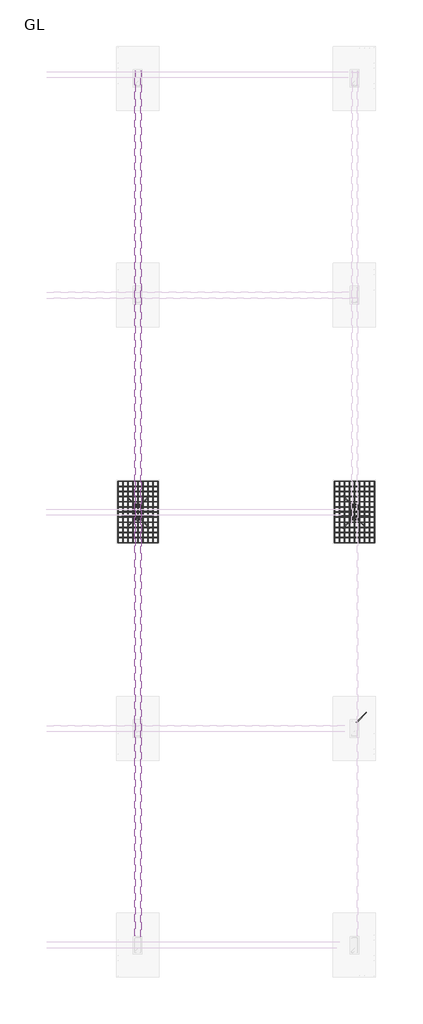
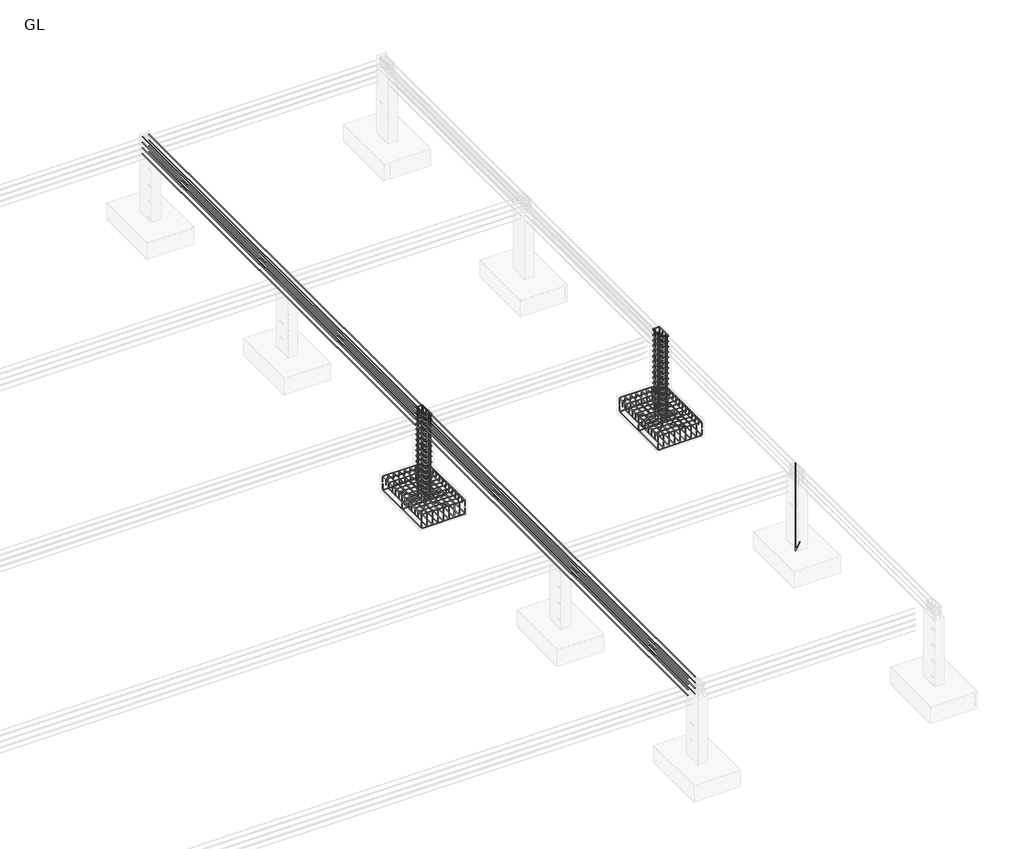
# One storey, part 12 of 16: 24 reinforcing bars.
"""IFC4 building model written with IfcOpenShell, lengths in millimetres."""

from ifc_helpers import new_model, si_unit, point, frame, origin, place, context, project, spatial, polyline, circle_curve, trimmed, segment, composite_curve, source, transform, mapped, element, save
from ifc_brep_helpers import swept_disk

model = new_model("IFC4")

# Units and contexts
model_context = context("Model", 3, world=origin())
ifc_project = project(units=[si_unit("LENGTHUNIT", "METRE", prefix="MILLI")], contexts=[model_context])

# Site, building, storey
site = spatial("IfcSite", under=ifc_project)
building = spatial("IfcBuilding", under=site)
storey = spatial("IfcBuildingStorey", under=building, Name="GL", Elevation=-1829.0)

# Reinforcing bars
placement = place(None, origin())
reinforcing_bar_shape = source(origin(), model_context, "Body", "SolidModel", [
    swept_disk(composite_curve([segment(polyline([(2141.0455621, -7223.1167521, -2089.0), (2141.0455621, -7223.1167521, -2213.0)]), True, "CONTINUOUS"), segment(trimmed(circle_curve(frame((2111.0455621, -7223.1167521, -2213.0), z_axis=(0.0, 1.0, 0.0), x_axis=(30.0, 0.0, 0.0)), 30.0), [point((2141.0455621, -7223.1167521, -2213.0))], [point((2111.0455621, -7223.1167521, -2243.0))], True, "CARTESIAN"), True, "CONTINUOUS"), segment(polyline([(2111.0455621, -7223.1167521, -2243.0), (1043.0455621, -7223.1167521, -2243.0)]), True, "CONTINUOUS"), segment(trimmed(circle_curve(frame((1043.0455621, -7223.1167521, -2213.0), z_axis=(0.0, 1.0, 0.0), x_axis=(0.0, 0.0, -30.0)), 30.0), [point((1043.0455621, -7223.1167521, -2243.0))], [point((1013.0455621, -7223.1167521, -2213.0))], True, "CARTESIAN"), True, "CONTINUOUS"), segment(polyline([(1013.0455621, -7223.1167521, -2213.0), (1013.0455621, -7223.1167521, -2089.0)]), True, "CONTINUOUS")], self_intersect=False), 6.0),
])
element("IfcReinforcingBar", 1, at=placement, inside=storey, context=model_context, shape_type="MappedRepresentation", body=[
    mapped(reinforcing_bar_shape, transform((0.0, 0.0, 0.0), x_axis=(1.0, 0.0, 0.0), y_axis=(0.0, 1.0, 0.0), z_axis=(0.0, 0.0, 1.0))),
    mapped(reinforcing_bar_shape, transform((0.0, -864.0, 0.0), x_axis=(1.0, 0.0, 0.0), y_axis=(0.0, 1.0, 0.0), z_axis=(0.0, 0.0, 1.0))),
    mapped(reinforcing_bar_shape, transform((0.0, -1728.0, 0.0), x_axis=(1.0, 0.0, 0.0), y_axis=(0.0, 1.0, 0.0), z_axis=(0.0, 0.0, 1.0))),
])
reinforcing_bar_2_shape = source(origin(), model_context, "Body", "SolidModel", [
    swept_disk(composite_curve([segment(polyline([(1013.0455621, -7223.1167521, -2022.436678), (1013.0455621, -7223.1167521, -1898.436678)]), True, "CONTINUOUS"), segment(trimmed(circle_curve(frame((1043.0455621, -7223.1167521, -1898.436678), z_axis=(0.0, 1.0, 0.0), x_axis=(-30.000000000000114, 0.0, 0.0)), 30.0), [point((1013.0455621, -7223.1167521, -1898.436678))], [point((1043.0455621, -7223.1167521, -1868.436678))], True, "CARTESIAN"), True, "CONTINUOUS"), segment(polyline([(1043.0455621, -7223.1167521, -1868.436678), (2111.0455621, -7223.1167521, -1868.436678)]), True, "CONTINUOUS"), segment(trimmed(circle_curve(frame((2111.0455621, -7223.1167521, -1898.436678), z_axis=(0.0, 1.0, 0.0), x_axis=(0.0, 0.0, 30.0)), 30.0), [point((2111.0455621, -7223.1167521, -1868.436678))], [point((2141.0455621, -7223.1167521, -1898.436678))], True, "CARTESIAN"), True, "CONTINUOUS"), segment(polyline([(2141.0455621, -7223.1167521, -1898.436678), (2141.0455621, -7223.1167521, -2022.436678)]), True, "CONTINUOUS")], self_intersect=False), 6.0),
])
element("IfcReinforcingBar", 2, at=placement, inside=storey, context=model_context, shape_type="MappedRepresentation", body=[
    mapped(reinforcing_bar_2_shape, transform((0.0, 0.0, 0.0), x_axis=(1.0, 0.0, 0.0), y_axis=(0.0, 1.0, 0.0), z_axis=(0.0, 0.0, 1.0))),
    mapped(reinforcing_bar_2_shape, transform((0.0, -144.0, 0.0), x_axis=(1.0, 0.0, 0.0), y_axis=(0.0, 1.0, 0.0), z_axis=(0.0, 0.0, 1.0))),
    mapped(reinforcing_bar_2_shape, transform((0.0, -288.0, 0.0), x_axis=(1.0, 0.0, 0.0), y_axis=(0.0, 1.0, 0.0), z_axis=(0.0, 0.0, 1.0))),
    mapped(reinforcing_bar_2_shape, transform((0.0, -432.0, 0.0), x_axis=(1.0, 0.0, 0.0), y_axis=(0.0, 1.0, 0.0), z_axis=(0.0, 0.0, 1.0))),
    mapped(reinforcing_bar_2_shape, transform((0.0, -576.0, 0.0), x_axis=(1.0, 0.0, 0.0), y_axis=(0.0, 1.0, 0.0), z_axis=(0.0, 0.0, 1.0))),
    mapped(reinforcing_bar_2_shape, transform((0.0, -720.0, 0.0), x_axis=(1.0, 0.0, 0.0), y_axis=(0.0, 1.0, 0.0), z_axis=(0.0, 0.0, 1.0))),
    mapped(reinforcing_bar_2_shape, transform((0.0, -864.0, 0.0), x_axis=(1.0, 0.0, 0.0), y_axis=(0.0, 1.0, 0.0), z_axis=(0.0, 0.0, 1.0))),
    mapped(reinforcing_bar_2_shape, transform((0.0, -1008.0, 0.0), x_axis=(1.0, 0.0, 0.0), y_axis=(0.0, 1.0, 0.0), z_axis=(0.0, 0.0, 1.0))),
    mapped(reinforcing_bar_2_shape, transform((0.0, -1152.0, 0.0), x_axis=(1.0, 0.0, 0.0), y_axis=(0.0, 1.0, 0.0), z_axis=(0.0, 0.0, 1.0))),
    mapped(reinforcing_bar_2_shape, transform((0.0, -1296.0, 0.0), x_axis=(1.0, 0.0, 0.0), y_axis=(0.0, 1.0, 0.0), z_axis=(0.0, 0.0, 1.0))),
    mapped(reinforcing_bar_2_shape, transform((0.0, -1440.0, 0.0), x_axis=(1.0, 0.0, 0.0), y_axis=(0.0, 1.0, 0.0), z_axis=(0.0, 0.0, 1.0))),
    mapped(reinforcing_bar_2_shape, transform((0.0, -1584.0, 0.0), x_axis=(1.0, 0.0, 0.0), y_axis=(0.0, 1.0, 0.0), z_axis=(0.0, 0.0, 1.0))),
    mapped(reinforcing_bar_2_shape, transform((0.0, -1728.0, 0.0), x_axis=(1.0, 0.0, 0.0), y_axis=(0.0, 1.0, 0.0), z_axis=(0.0, 0.0, 1.0))),
])
reinforcing_bar_3_shape = source(origin(), model_context, "Body", "SolidModel", [
    swept_disk(composite_curve([segment(polyline([(1013.0455621, -8951.1167521, -2027.5081232), (1013.0455621, -8951.1167521, -1903.5081232)]), True, "CONTINUOUS"), segment(trimmed(circle_curve(frame((1013.0455621, -8921.1167521, -1903.5081232), z_axis=(-1.0, 0.0, 0.0), x_axis=(0.0, -30.0, 0.0)), 30.0), [point((1013.0455621, -8951.1167521, -1903.5081232))], [point((1013.0455621, -8921.1167521, -1873.5081232))], True, "CARTESIAN"), True, "CONTINUOUS"), segment(polyline([(1013.0455621, -8921.1167521, -1873.5081232), (1013.0455621, -7253.1167521, -1873.5081232)]), True, "CONTINUOUS"), segment(trimmed(circle_curve(frame((1013.0455621, -7253.1167521, -1903.5081232), z_axis=(-1.0, 0.0, 0.0), x_axis=(0.0, 0.0, 30.0)), 30.0), [point((1013.0455621, -7253.1167521, -1873.5081232))], [point((1013.0455621, -7223.1167521, -1903.5081232))], True, "CARTESIAN"), True, "CONTINUOUS"), segment(polyline([(1013.0455621, -7223.1167521, -1903.5081232), (1013.0455621, -7223.1167521, -2027.5081232)]), True, "CONTINUOUS")], self_intersect=False), 6.0),
])
element("IfcReinforcingBar", 3, at=placement, inside=storey, context=model_context, shape_type="MappedRepresentation", body=[
    mapped(reinforcing_bar_3_shape, transform((0.0, 0.0, 0.0), x_axis=(1.0, 0.0, 0.0), y_axis=(0.0, 1.0, 0.0), z_axis=(0.0, 0.0, 1.0))),
    mapped(reinforcing_bar_3_shape, transform((141.0, 0.0, 0.0), x_axis=(1.0, 0.0, 0.0), y_axis=(0.0, 1.0, 0.0), z_axis=(0.0, 0.0, 1.0))),
    mapped(reinforcing_bar_3_shape, transform((282.0, 0.0, 0.0), x_axis=(1.0, 0.0, 0.0), y_axis=(0.0, 1.0, 0.0), z_axis=(0.0, 0.0, 1.0))),
    mapped(reinforcing_bar_3_shape, transform((423.0, 0.0, 0.0), x_axis=(1.0, 0.0, 0.0), y_axis=(0.0, 1.0, 0.0), z_axis=(0.0, 0.0, 1.0))),
    mapped(reinforcing_bar_3_shape, transform((564.0, 0.0, 0.0), x_axis=(1.0, 0.0, 0.0), y_axis=(0.0, 1.0, 0.0), z_axis=(0.0, 0.0, 1.0))),
    mapped(reinforcing_bar_3_shape, transform((705.0, 0.0, 0.0), x_axis=(1.0, 0.0, 0.0), y_axis=(0.0, 1.0, 0.0), z_axis=(0.0, 0.0, 1.0))),
    mapped(reinforcing_bar_3_shape, transform((846.0, 0.0, 0.0), x_axis=(1.0, 0.0, 0.0), y_axis=(0.0, 1.0, 0.0), z_axis=(0.0, 0.0, 1.0))),
    mapped(reinforcing_bar_3_shape, transform((987.0, 0.0, 0.0), x_axis=(1.0, 0.0, 0.0), y_axis=(0.0, 1.0, 0.0), z_axis=(0.0, 0.0, 1.0))),
    mapped(reinforcing_bar_3_shape, transform((1128.0, 0.0, 0.0), x_axis=(1.0, 0.0, 0.0), y_axis=(0.0, 1.0, 0.0), z_axis=(0.0, 0.0, 1.0))),
])
reinforcing_bar_4_shape = source(origin(), model_context, "Body", "SolidModel", [
    swept_disk(composite_curve([segment(polyline([(2141.0455621, -8951.1167521, -2080.6239909), (2141.0455621, -8951.1167521, -2204.6239909)]), True, "CONTINUOUS"), segment(trimmed(circle_curve(frame((2141.0455621, -8921.1167521, -2204.6239909), z_axis=(1.0, 0.0, 0.0), x_axis=(0.0, -30.0, 0.0)), 30.0), [point((2141.0455621, -8951.1167521, -2204.6239909))], [point((2141.0455621, -8921.1167521, -2234.6239909))], True, "CARTESIAN"), True, "CONTINUOUS"), segment(polyline([(2141.0455621, -8921.1167521, -2234.6239909), (2141.0455621, -7266.1421892, -2234.6239909)]), True, "CONTINUOUS"), segment(trimmed(circle_curve(frame((2141.0455621, -7266.1421892, -2204.6239909), z_axis=(1.0, 0.0, 0.0), x_axis=(0.0, 0.0, -30.0)), 30.0), [point((2141.0455621, -7266.1421892, -2234.6239909))], [point((2141.0455621, -7236.1421892, -2204.6239909))], True, "CARTESIAN"), True, "CONTINUOUS"), segment(polyline([(2141.0455621, -7236.1421892, -2204.6239909), (2141.0455621, -7236.1421892, -2080.6239909)]), True, "CONTINUOUS")], self_intersect=False), 6.0),
])
element("IfcReinforcingBar", 4, at=placement, inside=storey, context=model_context, shape_type="MappedRepresentation", body=[
    mapped(reinforcing_bar_4_shape, transform((0.0, 0.0, 0.0), x_axis=(1.0, 0.0, 0.0), y_axis=(0.0, 1.0, 0.0), z_axis=(0.0, 0.0, 1.0))),
    mapped(reinforcing_bar_4_shape, transform((-141.0, 0.0, 0.0), x_axis=(1.0, 0.0, 0.0), y_axis=(0.0, 1.0, 0.0), z_axis=(0.0, 0.0, 1.0))),
    mapped(reinforcing_bar_4_shape, transform((-282.0, 0.0, 0.0), x_axis=(1.0, 0.0, 0.0), y_axis=(0.0, 1.0, 0.0), z_axis=(0.0, 0.0, 1.0))),
    mapped(reinforcing_bar_4_shape, transform((-423.0, 0.0, 0.0), x_axis=(1.0, 0.0, 0.0), y_axis=(0.0, 1.0, 0.0), z_axis=(0.0, 0.0, 1.0))),
    mapped(reinforcing_bar_4_shape, transform((-564.0, 0.0, 0.0), x_axis=(1.0, 0.0, 0.0), y_axis=(0.0, 1.0, 0.0), z_axis=(0.0, 0.0, 1.0))),
    mapped(reinforcing_bar_4_shape, transform((-705.0, 0.0, 0.0), x_axis=(1.0, 0.0, 0.0), y_axis=(0.0, 1.0, 0.0), z_axis=(0.0, 0.0, 1.0))),
    mapped(reinforcing_bar_4_shape, transform((-846.0, 0.0, 0.0), x_axis=(1.0, 0.0, 0.0), y_axis=(0.0, 1.0, 0.0), z_axis=(0.0, 0.0, 1.0))),
    mapped(reinforcing_bar_4_shape, transform((-987.0, 0.0, 0.0), x_axis=(1.0, 0.0, 0.0), y_axis=(0.0, 1.0, 0.0), z_axis=(0.0, 0.0, 1.0))),
    mapped(reinforcing_bar_4_shape, transform((-1128.0, 0.0, 0.0), x_axis=(1.0, 0.0, 0.0), y_axis=(0.0, 1.0, 0.0), z_axis=(0.0, 0.0, 1.0))),
])
reinforcing_bar_5_shape = source(origin(), model_context, "Body", "SolidModel", [
    swept_disk(composite_curve([segment(polyline([(8237.0455621, -7223.1167521, -2089.0), (8237.0455621, -7223.1167521, -2213.0)]), True, "CONTINUOUS"), segment(trimmed(circle_curve(frame((8207.0455621, -7223.1167521, -2213.0), z_axis=(0.0, 1.0, 0.0), x_axis=(30.0, 0.0, 0.0)), 30.0), [point((8237.0455621, -7223.1167521, -2213.0))], [point((8207.0455621, -7223.1167521, -2243.0))], True, "CARTESIAN"), True, "CONTINUOUS"), segment(polyline([(8207.0455621, -7223.1167521, -2243.0), (7139.0455621, -7223.1167521, -2243.0)]), True, "CONTINUOUS"), segment(trimmed(circle_curve(frame((7139.0455621, -7223.1167521, -2213.0), z_axis=(0.0, 1.0, 0.0), x_axis=(0.0, 0.0, -30.0)), 30.0), [point((7139.0455621, -7223.1167521, -2243.0))], [point((7109.0455621, -7223.1167521, -2213.0))], True, "CARTESIAN"), True, "CONTINUOUS"), segment(polyline([(7109.0455621, -7223.1167521, -2213.0), (7109.0455621, -7223.1167521, -2089.0)]), True, "CONTINUOUS")], self_intersect=False), 6.0),
])
element("IfcReinforcingBar", 5, at=placement, inside=storey, context=model_context, shape_type="MappedRepresentation", body=[
    mapped(reinforcing_bar_5_shape, transform((0.0, 0.0, 0.0), x_axis=(1.0, 0.0, 0.0), y_axis=(0.0, 1.0, 0.0), z_axis=(0.0, 0.0, 1.0))),
    mapped(reinforcing_bar_5_shape, transform((0.0, -864.0, 0.0), x_axis=(1.0, 0.0, 0.0), y_axis=(0.0, 1.0, 0.0), z_axis=(0.0, 0.0, 1.0))),
    mapped(reinforcing_bar_5_shape, transform((0.0, -1728.0, 0.0), x_axis=(1.0, 0.0, 0.0), y_axis=(0.0, 1.0, 0.0), z_axis=(0.0, 0.0, 1.0))),
])
reinforcing_bar_6_shape = source(origin(), model_context, "Body", "SolidModel", [
    swept_disk(composite_curve([segment(polyline([(7109.0455621, -7223.1167521, -2022.436678), (7109.0455621, -7223.1167521, -1898.436678)]), True, "CONTINUOUS"), segment(trimmed(circle_curve(frame((7139.0455621, -7223.1167521, -1898.436678), z_axis=(0.0, 1.0, 0.0), x_axis=(-30.0, 0.0, 0.0)), 30.0), [point((7109.0455621, -7223.1167521, -1898.436678))], [point((7139.0455621, -7223.1167521, -1868.436678))], True, "CARTESIAN"), True, "CONTINUOUS"), segment(polyline([(7139.0455621, -7223.1167521, -1868.436678), (8207.0455621, -7223.1167521, -1868.436678)]), True, "CONTINUOUS"), segment(trimmed(circle_curve(frame((8207.0455621, -7223.1167521, -1898.436678), z_axis=(0.0, 1.0, 0.0), x_axis=(0.0, 0.0, 30.0)), 30.0), [point((8207.0455621, -7223.1167521, -1868.436678))], [point((8237.0455621, -7223.1167521, -1898.436678))], True, "CARTESIAN"), True, "CONTINUOUS"), segment(polyline([(8237.0455621, -7223.1167521, -1898.436678), (8237.0455621, -7223.1167521, -2022.436678)]), True, "CONTINUOUS")], self_intersect=False), 6.0),
])
element("IfcReinforcingBar", 6, at=placement, inside=storey, context=model_context, shape_type="MappedRepresentation", body=[
    mapped(reinforcing_bar_6_shape, transform((0.0, 0.0, 0.0), x_axis=(1.0, 0.0, 0.0), y_axis=(0.0, 1.0, 0.0), z_axis=(0.0, 0.0, 1.0))),
    mapped(reinforcing_bar_6_shape, transform((0.0, -144.0, 0.0), x_axis=(1.0, 0.0, 0.0), y_axis=(0.0, 1.0, 0.0), z_axis=(0.0, 0.0, 1.0))),
    mapped(reinforcing_bar_6_shape, transform((0.0, -288.0, 0.0), x_axis=(1.0, 0.0, 0.0), y_axis=(0.0, 1.0, 0.0), z_axis=(0.0, 0.0, 1.0))),
    mapped(reinforcing_bar_6_shape, transform((0.0, -432.0, 0.0), x_axis=(1.0, 0.0, 0.0), y_axis=(0.0, 1.0, 0.0), z_axis=(0.0, 0.0, 1.0))),
    mapped(reinforcing_bar_6_shape, transform((0.0, -576.0, 0.0), x_axis=(1.0, 0.0, 0.0), y_axis=(0.0, 1.0, 0.0), z_axis=(0.0, 0.0, 1.0))),
    mapped(reinforcing_bar_6_shape, transform((0.0, -720.0, 0.0), x_axis=(1.0, 0.0, 0.0), y_axis=(0.0, 1.0, 0.0), z_axis=(0.0, 0.0, 1.0))),
    mapped(reinforcing_bar_6_shape, transform((0.0, -864.0, 0.0), x_axis=(1.0, 0.0, 0.0), y_axis=(0.0, 1.0, 0.0), z_axis=(0.0, 0.0, 1.0))),
    mapped(reinforcing_bar_6_shape, transform((0.0, -1008.0, 0.0), x_axis=(1.0, 0.0, 0.0), y_axis=(0.0, 1.0, 0.0), z_axis=(0.0, 0.0, 1.0))),
    mapped(reinforcing_bar_6_shape, transform((0.0, -1152.0, 0.0), x_axis=(1.0, 0.0, 0.0), y_axis=(0.0, 1.0, 0.0), z_axis=(0.0, 0.0, 1.0))),
    mapped(reinforcing_bar_6_shape, transform((0.0, -1296.0, 0.0), x_axis=(1.0, 0.0, 0.0), y_axis=(0.0, 1.0, 0.0), z_axis=(0.0, 0.0, 1.0))),
    mapped(reinforcing_bar_6_shape, transform((0.0, -1440.0, 0.0), x_axis=(1.0, 0.0, 0.0), y_axis=(0.0, 1.0, 0.0), z_axis=(0.0, 0.0, 1.0))),
    mapped(reinforcing_bar_6_shape, transform((0.0, -1584.0, 0.0), x_axis=(1.0, 0.0, 0.0), y_axis=(0.0, 1.0, 0.0), z_axis=(0.0, 0.0, 1.0))),
    mapped(reinforcing_bar_6_shape, transform((0.0, -1728.0, 0.0), x_axis=(1.0, 0.0, 0.0), y_axis=(0.0, 1.0, 0.0), z_axis=(0.0, 0.0, 1.0))),
])
reinforcing_bar_7_shape = source(origin(), model_context, "Body", "SolidModel", [
    swept_disk(composite_curve([segment(polyline([(7109.0455621, -8951.1167521, -2027.5081232), (7109.0455621, -8951.1167521, -1903.5081232)]), True, "CONTINUOUS"), segment(trimmed(circle_curve(frame((7109.0455621, -8921.1167521, -1903.5081232), z_axis=(-1.0, 0.0, 0.0), x_axis=(0.0, -30.0, 0.0)), 30.0), [point((7109.0455621, -8951.1167521, -1903.5081232))], [point((7109.0455621, -8921.1167521, -1873.5081232))], True, "CARTESIAN"), True, "CONTINUOUS"), segment(polyline([(7109.0455621, -8921.1167521, -1873.5081232), (7109.0455621, -7253.1167521, -1873.5081232)]), True, "CONTINUOUS"), segment(trimmed(circle_curve(frame((7109.0455621, -7253.1167521, -1903.5081232), z_axis=(-1.0, 0.0, 0.0), x_axis=(0.0, 0.0, 30.0)), 30.0), [point((7109.0455621, -7253.1167521, -1873.5081232))], [point((7109.0455621, -7223.1167521, -1903.5081232))], True, "CARTESIAN"), True, "CONTINUOUS"), segment(polyline([(7109.0455621, -7223.1167521, -1903.5081232), (7109.0455621, -7223.1167521, -2027.5081232)]), True, "CONTINUOUS")], self_intersect=False), 6.0),
])
element("IfcReinforcingBar", 7, at=placement, inside=storey, context=model_context, shape_type="MappedRepresentation", body=[
    mapped(reinforcing_bar_7_shape, transform((0.0, 0.0, 0.0), x_axis=(1.0, 0.0, 0.0), y_axis=(0.0, 1.0, 0.0), z_axis=(0.0, 0.0, 1.0))),
    mapped(reinforcing_bar_7_shape, transform((141.0, 0.0, 0.0), x_axis=(1.0, 0.0, 0.0), y_axis=(0.0, 1.0, 0.0), z_axis=(0.0, 0.0, 1.0))),
    mapped(reinforcing_bar_7_shape, transform((282.0, 0.0, 0.0), x_axis=(1.0, 0.0, 0.0), y_axis=(0.0, 1.0, 0.0), z_axis=(0.0, 0.0, 1.0))),
    mapped(reinforcing_bar_7_shape, transform((423.0, 0.0, 0.0), x_axis=(1.0, 0.0, 0.0), y_axis=(0.0, 1.0, 0.0), z_axis=(0.0, 0.0, 1.0))),
    mapped(reinforcing_bar_7_shape, transform((564.0, 0.0, 0.0), x_axis=(1.0, 0.0, 0.0), y_axis=(0.0, 1.0, 0.0), z_axis=(0.0, 0.0, 1.0))),
    mapped(reinforcing_bar_7_shape, transform((705.0, 0.0, 0.0), x_axis=(1.0, 0.0, 0.0), y_axis=(0.0, 1.0, 0.0), z_axis=(0.0, 0.0, 1.0))),
    mapped(reinforcing_bar_7_shape, transform((846.0, 0.0, 0.0), x_axis=(1.0, 0.0, 0.0), y_axis=(0.0, 1.0, 0.0), z_axis=(0.0, 0.0, 1.0))),
    mapped(reinforcing_bar_7_shape, transform((987.0, 0.0, 0.0), x_axis=(1.0, 0.0, 0.0), y_axis=(0.0, 1.0, 0.0), z_axis=(0.0, 0.0, 1.0))),
    mapped(reinforcing_bar_7_shape, transform((1128.0, 0.0, 0.0), x_axis=(1.0, 0.0, 0.0), y_axis=(0.0, 1.0, 0.0), z_axis=(0.0, 0.0, 1.0))),
])
reinforcing_bar_8_shape = source(origin(), model_context, "Body", "SolidModel", [
    swept_disk(composite_curve([segment(polyline([(8237.0455621, -8951.1167521, -2080.6239909), (8237.0455621, -8951.1167521, -2204.6239909)]), True, "CONTINUOUS"), segment(trimmed(circle_curve(frame((8237.0455621, -8921.1167521, -2204.6239909), z_axis=(1.0, 0.0, 0.0), x_axis=(0.0, -30.0, 0.0)), 30.0), [point((8237.0455621, -8951.1167521, -2204.6239909))], [point((8237.0455621, -8921.1167521, -2234.6239909))], True, "CARTESIAN"), True, "CONTINUOUS"), segment(polyline([(8237.0455621, -8921.1167521, -2234.6239909), (8237.0455621, -7266.1421892, -2234.6239909)]), True, "CONTINUOUS"), segment(trimmed(circle_curve(frame((8237.0455621, -7266.1421892, -2204.6239909), z_axis=(1.0, 0.0, 0.0), x_axis=(0.0, 0.0, -30.0)), 30.0), [point((8237.0455621, -7266.1421892, -2234.6239909))], [point((8237.0455621, -7236.1421892, -2204.6239909))], True, "CARTESIAN"), True, "CONTINUOUS"), segment(polyline([(8237.0455621, -7236.1421892, -2204.6239909), (8237.0455621, -7236.1421892, -2080.6239909)]), True, "CONTINUOUS")], self_intersect=False), 6.0),
])
element("IfcReinforcingBar", 8, at=placement, inside=storey, context=model_context, shape_type="MappedRepresentation", body=[
    mapped(reinforcing_bar_8_shape, transform((0.0, 0.0, 0.0), x_axis=(1.0, 0.0, 0.0), y_axis=(0.0, 1.0, 0.0), z_axis=(0.0, 0.0, 1.0))),
    mapped(reinforcing_bar_8_shape, transform((-141.0, 0.0, 0.0), x_axis=(1.0, 0.0, 0.0), y_axis=(0.0, 1.0, 0.0), z_axis=(0.0, 0.0, 1.0))),
    mapped(reinforcing_bar_8_shape, transform((-282.0, 0.0, 0.0), x_axis=(1.0, 0.0, 0.0), y_axis=(0.0, 1.0, 0.0), z_axis=(0.0, 0.0, 1.0))),
    mapped(reinforcing_bar_8_shape, transform((-423.0, 0.0, 0.0), x_axis=(1.0, 0.0, 0.0), y_axis=(0.0, 1.0, 0.0), z_axis=(0.0, 0.0, 1.0))),
    mapped(reinforcing_bar_8_shape, transform((-564.0, 0.0, 0.0), x_axis=(1.0, 0.0, 0.0), y_axis=(0.0, 1.0, 0.0), z_axis=(0.0, 0.0, 1.0))),
    mapped(reinforcing_bar_8_shape, transform((-705.0, 0.0, 0.0), x_axis=(1.0, 0.0, 0.0), y_axis=(0.0, 1.0, 0.0), z_axis=(0.0, 0.0, 1.0))),
    mapped(reinforcing_bar_8_shape, transform((-846.0, 0.0, 0.0), x_axis=(1.0, 0.0, 0.0), y_axis=(0.0, 1.0, 0.0), z_axis=(0.0, 0.0, 1.0))),
    mapped(reinforcing_bar_8_shape, transform((-987.0, 0.0, 0.0), x_axis=(1.0, 0.0, 0.0), y_axis=(0.0, 1.0, 0.0), z_axis=(0.0, 0.0, 1.0))),
    mapped(reinforcing_bar_8_shape, transform((-1128.0, 0.0, 0.0), x_axis=(1.0, 0.0, 0.0), y_axis=(0.0, 1.0, 0.0), z_axis=(0.0, 0.0, 1.0))),
])
reinforcing_bar_9_shape = source(origin(), model_context, "Body", "SolidModel", [
    swept_disk(composite_curve([segment(polyline([(7680.5135995, -8162.2223078, -1793.0), (7592.8323586, -8249.9035486, -1793.0)]), True, "CONTINUOUS"), segment(trimmed(circle_curve(frame((7614.0455621, -8271.1167521, -1793.0), z_axis=(0.0, 0.0, 1.0), x_axis=(-21.213203500000418, 21.213203500001327, 0.0)), 30.0), [point((7592.8323586, -8249.9035486, -1793.0))], [point((7614.0455621, -8301.1167521, -1793.0))], True, "CARTESIAN"), True, "CONTINUOUS"), segment(polyline([(7614.0455621, -8301.1167521, -1793.0), (7732.0455621, -8301.1167521, -1793.0)]), True, "CONTINUOUS"), segment(trimmed(circle_curve(frame((7732.0455621, -8271.1167521, -1793.0), z_axis=(0.0, 0.0, 1.0), x_axis=(0.0, -30.0, 0.0)), 30.0), [point((7732.0455621, -8301.1167521, -1793.0))], [point((7762.0455621, -8271.1167521, -1793.0))], True, "CARTESIAN"), True, "CONTINUOUS"), segment(polyline([(7762.0455621, -8271.1167521, -1793.0), (7762.0455621, -7903.1167521, -1793.0)]), True, "CONTINUOUS"), segment(trimmed(circle_curve(frame((7732.1135038, -7903.1167521, -1795.0178916), z_axis=(-0.06726305234213417, 0.0, 0.9977352764083365), x_axis=(29.93205829999988, 0.0, 2.0178915999999845)), 30.0), [point((7762.0455621, -7903.1167521, -1793.0))], [point((7732.1135038, -7873.1167521, -1795.0178916))], True, "CARTESIAN"), True, "CONTINUOUS"), segment(polyline([(7732.1135038, -7873.1167521, -1795.0178916), (7613.9776204, -7873.1167521, -1802.9821084)]), True, "CONTINUOUS"), segment(trimmed(circle_curve(frame((7613.9776204, -7903.1167521, -1802.9821084), z_axis=(-0.06726305234213417, 0.0, 0.9977352764083365), x_axis=(0.0, 30.0, 0.0)), 30.0), [point((7613.9776204, -7873.1167521, -1802.9821084))], [point((7584.0455621, -7903.1167521, -1805.0))], True, "CARTESIAN"), True, "CONTINUOUS"), segment(polyline([(7584.0455621, -7903.1167521, -1805.0), (7584.0455621, -8271.1167521, -1805.0)]), True, "CONTINUOUS"), segment(trimmed(circle_curve(frame((7614.0455621, -8271.1167521, -1805.0), z_axis=(0.0, 0.0, 1.0), x_axis=(-30.0, 0.0, 0.0)), 30.0), [point((7584.0455621, -8271.1167521, -1805.0))], [point((7635.2587655, -8292.3299555, -1805.0))], True, "CARTESIAN"), True, "CONTINUOUS"), segment(polyline([(7635.2587655, -8292.3299555, -1805.0), (7722.9400064, -8204.6487146, -1805.0)]), True, "CONTINUOUS")], self_intersect=False), 6.0),
])
element("IfcReinforcingBar", 9, at=placement, inside=storey, context=model_context, shape_type="MappedRepresentation", body=[
    mapped(reinforcing_bar_9_shape, transform((0.0, 0.0, 0.0), x_axis=(1.0, 0.0, 0.0), y_axis=(0.0, 1.0, 0.0), z_axis=(0.0, 0.0, 1.0))),
    mapped(reinforcing_bar_9_shape, transform((0.0, 0.0, 144.8571429), x_axis=(1.0, 0.0, 0.0), y_axis=(0.0, 1.0, 0.0), z_axis=(0.0, 0.0, 1.0))),
    mapped(reinforcing_bar_9_shape, transform((0.0, 0.0, 289.7142857), x_axis=(1.0, 0.0, 0.0), y_axis=(0.0, 1.0, 0.0), z_axis=(0.0, 0.0, 1.0))),
    mapped(reinforcing_bar_9_shape, transform((0.0, 0.0, 434.5714286), x_axis=(1.0, 0.0, 0.0), y_axis=(0.0, 1.0, 0.0), z_axis=(0.0, 0.0, 1.0))),
    mapped(reinforcing_bar_9_shape, transform((0.0, 0.0, 579.4285714), x_axis=(1.0, 0.0, 0.0), y_axis=(0.0, 1.0, 0.0), z_axis=(0.0, 0.0, 1.0))),
    mapped(reinforcing_bar_9_shape, transform((0.0, 0.0, 724.2857143), x_axis=(1.0, 0.0, 0.0), y_axis=(0.0, 1.0, 0.0), z_axis=(0.0, 0.0, 1.0))),
    mapped(reinforcing_bar_9_shape, transform((0.0, 0.0, 869.1428571), x_axis=(1.0, 0.0, 0.0), y_axis=(0.0, 1.0, 0.0), z_axis=(0.0, 0.0, 1.0))),
    mapped(reinforcing_bar_9_shape, transform((0.0, 0.0, 1014.0), x_axis=(1.0, 0.0, 0.0), y_axis=(0.0, 1.0, 0.0), z_axis=(0.0, 0.0, 1.0))),
    mapped(reinforcing_bar_9_shape, transform((0.0, 0.0, 1158.8571429), x_axis=(1.0, 0.0, 0.0), y_axis=(0.0, 1.0, 0.0), z_axis=(0.0, 0.0, 1.0))),
    mapped(reinforcing_bar_9_shape, transform((0.0, 0.0, 1303.7142857), x_axis=(1.0, 0.0, 0.0), y_axis=(0.0, 1.0, 0.0), z_axis=(0.0, 0.0, 1.0))),
    mapped(reinforcing_bar_9_shape, transform((0.0, 0.0, 1448.5714286), x_axis=(1.0, 0.0, 0.0), y_axis=(0.0, 1.0, 0.0), z_axis=(0.0, 0.0, 1.0))),
    mapped(reinforcing_bar_9_shape, transform((0.0, 0.0, 1593.4285714), x_axis=(1.0, 0.0, 0.0), y_axis=(0.0, 1.0, 0.0), z_axis=(0.0, 0.0, 1.0))),
    mapped(reinforcing_bar_9_shape, transform((0.0, 0.0, 1738.2857143), x_axis=(1.0, 0.0, 0.0), y_axis=(0.0, 1.0, 0.0), z_axis=(0.0, 0.0, 1.0))),
    mapped(reinforcing_bar_9_shape, transform((0.0, 0.0, 1883.1428571), x_axis=(1.0, 0.0, 0.0), y_axis=(0.0, 1.0, 0.0), z_axis=(0.0, 0.0, 1.0))),
    mapped(reinforcing_bar_9_shape, transform((0.0, 0.0, 2028.0), x_axis=(1.0, 0.0, 0.0), y_axis=(0.0, 1.0, 0.0), z_axis=(0.0, 0.0, 1.0))),
])
element("IfcReinforcingBar", 10, at=placement, inside=storey, context=model_context, shape_type="SolidModel", body=[
    swept_disk(composite_curve([segment(polyline([(7615.9357768, -8272.0642439, 241.0), (7615.9357768, -8272.0642439, -2129.0)]), True, "CONTINUOUS"), segment(trimmed(circle_curve(frame((7594.7225734, -8293.2774473, -2129.0), z_axis=(-0.7071067811865187, 0.7071067811865764, 0.0), x_axis=(21.213203399999657, 21.213203400000566, 0.0)), 30.0), [point((7615.9357768, -8272.0642439, -2129.0))], [point((7594.7225734, -8293.2774473, -2159.0))], True, "CARTESIAN"), True, "CONTINUOUS"), segment(polyline([(7594.7225734, -8293.2774473, -2159.0), (7347.2352, -8540.7648207, -2159.0)]), True, "CONTINUOUS")], self_intersect=False), 6.0),
])
element("IfcReinforcingBar", 11, at=placement, inside=storey, context=model_context, shape_type="SolidModel", body=[
    swept_disk(composite_curve([segment(polyline([(7615.9357768, -7902.1692603, 241.0), (7615.9357768, -7902.1692603, -2129.0)]), True, "CONTINUOUS"), segment(trimmed(circle_curve(frame((7594.7225734, -7880.9560568, -2129.0), z_axis=(0.7071067811865218, 0.7071067811865733, 0.0), x_axis=(21.213203399999657, -21.213203500000418, 0.0)), 30.0), [point((7615.9357768, -7902.1692603, -2129.0))], [point((7594.7225734, -7880.9560568, -2159.0))], True, "CARTESIAN"), True, "CONTINUOUS"), segment(polyline([(7594.7225734, -7880.9560568, -2159.0), (7347.2352, -7633.4686834, -2159.0)]), True, "CONTINUOUS")], self_intersect=False), 6.0),
])
element("IfcReinforcingBar", 12, at=placement, inside=storey, context=model_context, shape_type="SolidModel", body=[
    swept_disk(composite_curve([segment(polyline([(7730.1553473, -8272.0642439, 241.0), (7730.1553473, -8272.0642439, -2129.0)]), True, "CONTINUOUS"), segment(trimmed(circle_curve(frame((7751.3685508, -8293.2774473, -2129.0), z_axis=(-0.7071067811865248, -0.7071067811865703, 0.0), x_axis=(-21.21320349999951, 21.213203400000566, 0.0)), 30.0), [point((7730.1553473, -8272.0642439, -2129.0))], [point((7751.3685508, -8293.2774473, -2159.0))], True, "CARTESIAN"), True, "CONTINUOUS"), segment(polyline([(7751.3685508, -8293.2774473, -2159.0), (7998.8559242, -8540.7648207, -2159.0)]), True, "CONTINUOUS")], self_intersect=False), 6.0),
])
reinforcing_bar_10_shape = source(origin(), model_context, "Body", "SolidModel", [
    swept_disk(composite_curve([segment(polyline([(7615.9357768, -8194.9117405, 241.0), (7615.9357768, -8194.9117405, -2129.0)]), True, "CONTINUOUS"), segment(trimmed(circle_curve(frame((7585.9357768, -8194.9117405, -2129.0), z_axis=(0.0, 1.0, 0.0), x_axis=(30.0, 0.0, 0.0)), 30.0), [point((7615.9357768, -8194.9117405, -2129.0))], [point((7585.9357768, -8194.9117405, -2159.0))], True, "CARTESIAN"), True, "CONTINUOUS"), segment(polyline([(7585.9357768, -8194.9117405, -2159.0), (7235.9357768, -8194.9117405, -2159.0)]), True, "CONTINUOUS")], self_intersect=False), 6.0),
])
element("IfcReinforcingBar", 13, at=placement, inside=storey, context=model_context, shape_type="MappedRepresentation", body=[
    mapped(reinforcing_bar_10_shape, transform((0.0, 0.0, 0.0), x_axis=(1.0, 0.0, 0.0), y_axis=(0.0, 1.0, 0.0), z_axis=(0.0, 0.0, 1.0))),
    mapped(reinforcing_bar_10_shape, transform((0.0, 123.5823926, 0.0), x_axis=(1.0, 0.0, 0.0), y_axis=(0.0, 1.0, 0.0), z_axis=(0.0, 0.0, 1.0))),
    mapped(reinforcing_bar_10_shape, transform((0.0, 247.1647853, 0.0), x_axis=(1.0, 0.0, 0.0), y_axis=(0.0, 1.0, 0.0), z_axis=(0.0, 0.0, 1.0))),
])
reinforcing_bar_11_shape = source(origin(), model_context, "Body", "SolidModel", [
    swept_disk(composite_curve([segment(polyline([(7730.1553473, -8194.9117405, 241.0), (7730.1553473, -8194.9117405, -2129.0)]), True, "CONTINUOUS"), segment(trimmed(circle_curve(frame((7760.1553473, -8194.9117405, -2129.0), z_axis=(0.0, -1.0, 0.0), x_axis=(-30.0, 0.0, 0.0)), 30.0), [point((7730.1553473, -8194.9117405, -2129.0))], [point((7760.1553473, -8194.9117405, -2159.0))], True, "CARTESIAN"), True, "CONTINUOUS"), segment(polyline([(7760.1553473, -8194.9117405, -2159.0), (8110.1553473, -8194.9117405, -2159.0)]), True, "CONTINUOUS")], self_intersect=False), 6.0),
])
element("IfcReinforcingBar", 14, at=placement, inside=storey, context=model_context, shape_type="MappedRepresentation", body=[
    mapped(reinforcing_bar_11_shape, transform((0.0, 0.0, 0.0), x_axis=(1.0, 0.0, 0.0), y_axis=(0.0, 1.0, 0.0), z_axis=(0.0, 0.0, 1.0))),
    mapped(reinforcing_bar_11_shape, transform((0.0, 123.5823926, 0.0), x_axis=(1.0, 0.0, 0.0), y_axis=(0.0, 1.0, 0.0), z_axis=(0.0, 0.0, 1.0))),
    mapped(reinforcing_bar_11_shape, transform((0.0, 247.1647853, 0.0), x_axis=(1.0, 0.0, 0.0), y_axis=(0.0, 1.0, 0.0), z_axis=(0.0, 0.0, 1.0))),
])
element("IfcReinforcingBar", 15, at=placement, inside=storey, context=model_context, shape_type="SolidModel", body=[
    swept_disk(composite_curve([segment(polyline([(7730.1553473, -13998.1692603, 241.0), (7730.1553473, -13998.1692603, -2129.0)]), True, "CONTINUOUS"), segment(trimmed(circle_curve(frame((7751.3685508, -13976.9560568, -2129.0), z_axis=(0.7071067811865157, -0.7071067811865794, 0.0), x_axis=(-21.21320349999951, -21.21320349999951, 0.0)), 30.0), [point((7730.1553473, -13998.1692603, -2129.0))], [point((7751.3685508, -13976.9560568, -2159.0))], True, "CARTESIAN"), True, "CONTINUOUS"), segment(polyline([(7751.3685508, -13976.9560568, -2159.0), (7998.8559242, -13729.4686834, -2159.0)]), True, "CONTINUOUS")], self_intersect=False), 6.0),
])
reinforcing_bar_12_shape = source(origin(), model_context, "Body", "SolidModel", [
    swept_disk(composite_curve([segment(polyline([(1584.5135995, -8162.2223078, -1793.0), (1496.8323586, -8249.9035486, -1793.0)]), True, "CONTINUOUS"), segment(trimmed(circle_curve(frame((1518.0455621, -8271.1167521, -1793.0), z_axis=(0.0, 0.0, 1.0), x_axis=(-21.21320350000019, 21.213203500001327, 0.0)), 30.0), [point((1496.8323586, -8249.9035486, -1793.0))], [point((1518.0455621, -8301.1167521, -1793.0))], True, "CARTESIAN"), True, "CONTINUOUS"), segment(polyline([(1518.0455621, -8301.1167521, -1793.0), (1636.0455621, -8301.1167521, -1793.0)]), True, "CONTINUOUS"), segment(trimmed(circle_curve(frame((1636.0455621, -8271.1167521, -1793.0), z_axis=(0.0, 0.0, 1.0), x_axis=(0.0, -30.0, 0.0)), 30.0), [point((1636.0455621, -8301.1167521, -1793.0))], [point((1666.0455621, -8271.1167521, -1793.0))], True, "CARTESIAN"), True, "CONTINUOUS"), segment(polyline([(1666.0455621, -8271.1167521, -1793.0), (1666.0455621, -7903.1167521, -1793.0)]), True, "CONTINUOUS"), segment(trimmed(circle_curve(frame((1636.1135038, -7903.1167521, -1795.0178916), z_axis=(-0.06726305234213417, 0.0, 0.9977352764083365), x_axis=(29.932058300000108, 0.0, 2.0178915999999845)), 30.0), [point((1666.0455621, -7903.1167521, -1793.0))], [point((1636.1135038, -7873.1167521, -1795.0178916))], True, "CARTESIAN"), True, "CONTINUOUS"), segment(polyline([(1636.1135038, -7873.1167521, -1795.0178916), (1517.9776204, -7873.1167521, -1802.9821084)]), True, "CONTINUOUS"), segment(trimmed(circle_curve(frame((1517.9776204, -7903.1167521, -1802.9821084), z_axis=(-0.06726305234213417, 0.0, 0.9977352764083365), x_axis=(0.0, 30.0, 0.0)), 30.0), [point((1517.9776204, -7873.1167521, -1802.9821084))], [point((1488.0455621, -7903.1167521, -1805.0))], True, "CARTESIAN"), True, "CONTINUOUS"), segment(polyline([(1488.0455621, -7903.1167521, -1805.0), (1488.0455621, -8271.1167521, -1805.0)]), True, "CONTINUOUS"), segment(trimmed(circle_curve(frame((1518.0455621, -8271.1167521, -1805.0), z_axis=(0.0, 0.0, 1.0), x_axis=(-30.0, 0.0, 0.0)), 30.0), [point((1488.0455621, -8271.1167521, -1805.0))], [point((1539.2587655, -8292.3299555, -1805.0))], True, "CARTESIAN"), True, "CONTINUOUS"), segment(polyline([(1539.2587655, -8292.3299555, -1805.0), (1626.9400064, -8204.6487146, -1805.0)]), True, "CONTINUOUS")], self_intersect=False), 6.0),
])
element("IfcReinforcingBar", 16, at=placement, inside=storey, context=model_context, shape_type="MappedRepresentation", body=[
    mapped(reinforcing_bar_12_shape, transform((0.0, 0.0, 0.0), x_axis=(1.0, 0.0, 0.0), y_axis=(0.0, 1.0, 0.0), z_axis=(0.0, 0.0, 1.0))),
    mapped(reinforcing_bar_12_shape, transform((0.0, 0.0, 144.8571429), x_axis=(1.0, 0.0, 0.0), y_axis=(0.0, 1.0, 0.0), z_axis=(0.0, 0.0, 1.0))),
    mapped(reinforcing_bar_12_shape, transform((0.0, 0.0, 289.7142857), x_axis=(1.0, 0.0, 0.0), y_axis=(0.0, 1.0, 0.0), z_axis=(0.0, 0.0, 1.0))),
    mapped(reinforcing_bar_12_shape, transform((0.0, 0.0, 434.5714286), x_axis=(1.0, 0.0, 0.0), y_axis=(0.0, 1.0, 0.0), z_axis=(0.0, 0.0, 1.0))),
    mapped(reinforcing_bar_12_shape, transform((0.0, 0.0, 579.4285714), x_axis=(1.0, 0.0, 0.0), y_axis=(0.0, 1.0, 0.0), z_axis=(0.0, 0.0, 1.0))),
    mapped(reinforcing_bar_12_shape, transform((0.0, 0.0, 724.2857143), x_axis=(1.0, 0.0, 0.0), y_axis=(0.0, 1.0, 0.0), z_axis=(0.0, 0.0, 1.0))),
    mapped(reinforcing_bar_12_shape, transform((0.0, 0.0, 869.1428571), x_axis=(1.0, 0.0, 0.0), y_axis=(0.0, 1.0, 0.0), z_axis=(0.0, 0.0, 1.0))),
    mapped(reinforcing_bar_12_shape, transform((0.0, 0.0, 1014.0), x_axis=(1.0, 0.0, 0.0), y_axis=(0.0, 1.0, 0.0), z_axis=(0.0, 0.0, 1.0))),
    mapped(reinforcing_bar_12_shape, transform((0.0, 0.0, 1158.8571429), x_axis=(1.0, 0.0, 0.0), y_axis=(0.0, 1.0, 0.0), z_axis=(0.0, 0.0, 1.0))),
    mapped(reinforcing_bar_12_shape, transform((0.0, 0.0, 1303.7142857), x_axis=(1.0, 0.0, 0.0), y_axis=(0.0, 1.0, 0.0), z_axis=(0.0, 0.0, 1.0))),
    mapped(reinforcing_bar_12_shape, transform((0.0, 0.0, 1448.5714286), x_axis=(1.0, 0.0, 0.0), y_axis=(0.0, 1.0, 0.0), z_axis=(0.0, 0.0, 1.0))),
    mapped(reinforcing_bar_12_shape, transform((0.0, 0.0, 1593.4285714), x_axis=(1.0, 0.0, 0.0), y_axis=(0.0, 1.0, 0.0), z_axis=(0.0, 0.0, 1.0))),
    mapped(reinforcing_bar_12_shape, transform((0.0, 0.0, 1738.2857143), x_axis=(1.0, 0.0, 0.0), y_axis=(0.0, 1.0, 0.0), z_axis=(0.0, 0.0, 1.0))),
    mapped(reinforcing_bar_12_shape, transform((0.0, 0.0, 1883.1428571), x_axis=(1.0, 0.0, 0.0), y_axis=(0.0, 1.0, 0.0), z_axis=(0.0, 0.0, 1.0))),
    mapped(reinforcing_bar_12_shape, transform((0.0, 0.0, 2028.0), x_axis=(1.0, 0.0, 0.0), y_axis=(0.0, 1.0, 0.0), z_axis=(0.0, 0.0, 1.0))),
])
element("IfcReinforcingBar", 17, at=placement, inside=storey, context=model_context, shape_type="SolidModel", body=[
    swept_disk(composite_curve([segment(polyline([(1519.9357768, -8272.0642439, 241.0), (1519.9357768, -8272.0642439, -2129.0)]), True, "CONTINUOUS"), segment(trimmed(circle_curve(frame((1498.7225734, -8293.2774473, -2129.0), z_axis=(-0.7071067811865187, 0.7071067811865764, 0.0), x_axis=(21.213203399999884, 21.213203400000566, 0.0)), 30.0), [point((1519.9357768, -8272.0642439, -2129.0))], [point((1498.7225734, -8293.2774473, -2159.0))], True, "CARTESIAN"), True, "CONTINUOUS"), segment(polyline([(1498.7225734, -8293.2774473, -2159.0), (1251.2352, -8540.7648207, -2159.0)]), True, "CONTINUOUS")], self_intersect=False), 6.0),
])
element("IfcReinforcingBar", 18, at=placement, inside=storey, context=model_context, shape_type="SolidModel", body=[
    swept_disk(composite_curve([segment(polyline([(1519.9357768, -7902.1692603, 241.0), (1519.9357768, -7902.1692603, -2129.0)]), True, "CONTINUOUS"), segment(trimmed(circle_curve(frame((1498.7225734, -7880.9560568, -2129.0), z_axis=(0.7071067811865218, 0.7071067811865733, 0.0), x_axis=(21.213203399999884, -21.213203500000418, 0.0)), 30.0), [point((1519.9357768, -7902.1692603, -2129.0))], [point((1498.7225734, -7880.9560568, -2159.0))], True, "CARTESIAN"), True, "CONTINUOUS"), segment(polyline([(1498.7225734, -7880.9560568, -2159.0), (1251.2352, -7633.4686834, -2159.0)]), True, "CONTINUOUS")], self_intersect=False), 6.0),
])
element("IfcReinforcingBar", 19, at=placement, inside=storey, context=model_context, shape_type="SolidModel", body=[
    swept_disk(composite_curve([segment(polyline([(1634.1553473, -8272.0642439, 241.0), (1634.1553473, -8272.0642439, -2129.0)]), True, "CONTINUOUS"), segment(trimmed(circle_curve(frame((1655.3685508, -8293.2774473, -2129.0), z_axis=(-0.7071067811865248, -0.7071067811865703, 0.0), x_axis=(-21.21320350000019, 21.213203400000566, 0.0)), 30.0), [point((1634.1553473, -8272.0642439, -2129.0))], [point((1655.3685508, -8293.2774473, -2159.0))], True, "CARTESIAN"), True, "CONTINUOUS"), segment(polyline([(1655.3685508, -8293.2774473, -2159.0), (1902.8559242, -8540.7648207, -2159.0)]), True, "CONTINUOUS")], self_intersect=False), 6.0),
])
element("IfcReinforcingBar", 20, at=placement, inside=storey, context=model_context, shape_type="SolidModel", body=[
    swept_disk(composite_curve([segment(polyline([(1634.1553473, -7902.1692603, 241.0), (1634.1553473, -7902.1692603, -2129.0)]), True, "CONTINUOUS"), segment(trimmed(circle_curve(frame((1655.3685508, -7880.9560568, -2129.0), z_axis=(0.7071067811865157, -0.7071067811865794, 0.0), x_axis=(-21.21320350000019, -21.213203500000418, 0.0)), 30.0), [point((1634.1553473, -7902.1692603, -2129.0))], [point((1655.3685508, -7880.9560568, -2159.0))], True, "CARTESIAN"), True, "CONTINUOUS"), segment(polyline([(1655.3685508, -7880.9560568, -2159.0), (1902.8559242, -7633.4686834, -2159.0)]), True, "CONTINUOUS")], self_intersect=False), 6.0),
])
reinforcing_bar_13_shape = source(origin(), model_context, "Body", "SolidModel", [
    swept_disk(composite_curve([segment(polyline([(1519.9357768, -8194.9117405, 241.0), (1519.9357768, -8194.9117405, -2129.0)]), True, "CONTINUOUS"), segment(trimmed(circle_curve(frame((1489.9357768, -8194.9117405, -2129.0), z_axis=(0.0, 1.0, 0.0), x_axis=(30.0, 0.0, 0.0)), 30.0), [point((1519.9357768, -8194.9117405, -2129.0))], [point((1489.9357768, -8194.9117405, -2159.0))], True, "CARTESIAN"), True, "CONTINUOUS"), segment(polyline([(1489.9357768, -8194.9117405, -2159.0), (1139.9357768, -8194.9117405, -2159.0)]), True, "CONTINUOUS")], self_intersect=False), 6.0),
])
element("IfcReinforcingBar", 21, at=placement, inside=storey, context=model_context, shape_type="MappedRepresentation", body=[
    mapped(reinforcing_bar_13_shape, transform((0.0, 0.0, 0.0), x_axis=(1.0, 0.0, 0.0), y_axis=(0.0, 1.0, 0.0), z_axis=(0.0, 0.0, 1.0))),
    mapped(reinforcing_bar_13_shape, transform((0.0, 123.5823926, 0.0), x_axis=(1.0, 0.0, 0.0), y_axis=(0.0, 1.0, 0.0), z_axis=(0.0, 0.0, 1.0))),
    mapped(reinforcing_bar_13_shape, transform((0.0, 247.1647853, 0.0), x_axis=(1.0, 0.0, 0.0), y_axis=(0.0, 1.0, 0.0), z_axis=(0.0, 0.0, 1.0))),
])
reinforcing_bar_14_shape = source(origin(), model_context, "Body", "SolidModel", [
    swept_disk(composite_curve([segment(polyline([(1634.1553473, -8194.9117405, 241.0), (1634.1553473, -8194.9117405, -2129.0)]), True, "CONTINUOUS"), segment(trimmed(circle_curve(frame((1664.1553473, -8194.9117405, -2129.0), z_axis=(0.0, -1.0, 0.0), x_axis=(-30.0, 0.0, 0.0)), 30.0), [point((1634.1553473, -8194.9117405, -2129.0))], [point((1664.1553473, -8194.9117405, -2159.0))], True, "CARTESIAN"), True, "CONTINUOUS"), segment(polyline([(1664.1553473, -8194.9117405, -2159.0), (2014.1553473, -8194.9117405, -2159.0)]), True, "CONTINUOUS")], self_intersect=False), 6.0),
])
element("IfcReinforcingBar", 22, at=placement, inside=storey, context=model_context, shape_type="MappedRepresentation", body=[
    mapped(reinforcing_bar_14_shape, transform((0.0, 0.0, 0.0), x_axis=(1.0, 0.0, 0.0), y_axis=(0.0, 1.0, 0.0), z_axis=(0.0, 0.0, 1.0))),
    mapped(reinforcing_bar_14_shape, transform((0.0, 123.5823926, 0.0), x_axis=(1.0, 0.0, 0.0), y_axis=(0.0, 1.0, 0.0), z_axis=(0.0, 0.0, 1.0))),
    mapped(reinforcing_bar_14_shape, transform((0.0, 247.1647853, 0.0), x_axis=(1.0, 0.0, 0.0), y_axis=(0.0, 1.0, 0.0), z_axis=(0.0, 0.0, 1.0))),
])
reinforcing_bar_15_shape = source(origin(), model_context, "Body", "SolidModel", [
    swept_disk(composite_curve([segment(polyline([(1493.0455621, 4324.8832479, 208.5611075), (1493.0455621, -20006.0339034, 208.5611075)]), True, "CONTINUOUS")], self_intersect=False), 6.0),
])
element("IfcReinforcingBar", 23, at=placement, inside=storey, context=model_context, shape_type="MappedRepresentation", body=[
    mapped(reinforcing_bar_15_shape, transform((0.0, 0.0, 0.0), x_axis=(1.0, 0.0, 0.0), y_axis=(0.0, 1.0, 0.0), z_axis=(0.0, 0.0, 1.0))),
    mapped(reinforcing_bar_15_shape, transform((0.0, 0.0, -155.8763228), x_axis=(1.0, 0.0, 0.0), y_axis=(0.0, 1.0, 0.0), z_axis=(0.0, 0.0, 1.0))),
    mapped(reinforcing_bar_15_shape, transform((0.0, 0.0, -311.7526457), x_axis=(1.0, 0.0, 0.0), y_axis=(0.0, 1.0, 0.0), z_axis=(0.0, 0.0, 1.0))),
    mapped(reinforcing_bar_15_shape, transform((0.0, 0.0, -467.6289685), x_axis=(1.0, 0.0, 0.0), y_axis=(0.0, 1.0, 0.0), z_axis=(0.0, 0.0, 1.0))),
])
reinforcing_bar_16_shape = source(origin(), model_context, "Body", "SolidModel", [
    swept_disk(composite_curve([segment(polyline([(1661.0455621, 4324.8832479, -259.067861), (1661.0455621, -20031.8547975, -259.067861)]), True, "CONTINUOUS")], self_intersect=False), 6.0),
])
element("IfcReinforcingBar", 24, at=placement, inside=storey, context=model_context, shape_type="MappedRepresentation", body=[
    mapped(reinforcing_bar_16_shape, transform((0.0, 0.0, 0.0), x_axis=(1.0, 0.0, 0.0), y_axis=(0.0, 1.0, 0.0), z_axis=(0.0, 0.0, 1.0))),
    mapped(reinforcing_bar_16_shape, transform((0.0, 0.0, 155.8763228), x_axis=(1.0, 0.0, 0.0), y_axis=(0.0, 1.0, 0.0), z_axis=(0.0, 0.0, 1.0))),
    mapped(reinforcing_bar_16_shape, transform((0.0, 0.0, 311.7526457), x_axis=(1.0, 0.0, 0.0), y_axis=(0.0, 1.0, 0.0), z_axis=(0.0, 0.0, 1.0))),
    mapped(reinforcing_bar_16_shape, transform((0.0, 0.0, 467.6289685), x_axis=(1.0, 0.0, 0.0), y_axis=(0.0, 1.0, 0.0), z_axis=(0.0, 0.0, 1.0))),
])

save(model, "model.ifc")

# Revit data of these elements
# Elements 1, 2, 3, 4, 5, 6, 7, 8, 9, 10, 11, 12, 13, 14, 15, 16, 17, 18, 19, 20, 21, 22, 23, 24 (IfcReinforcingBar)
#   Phase Created = New Construction
